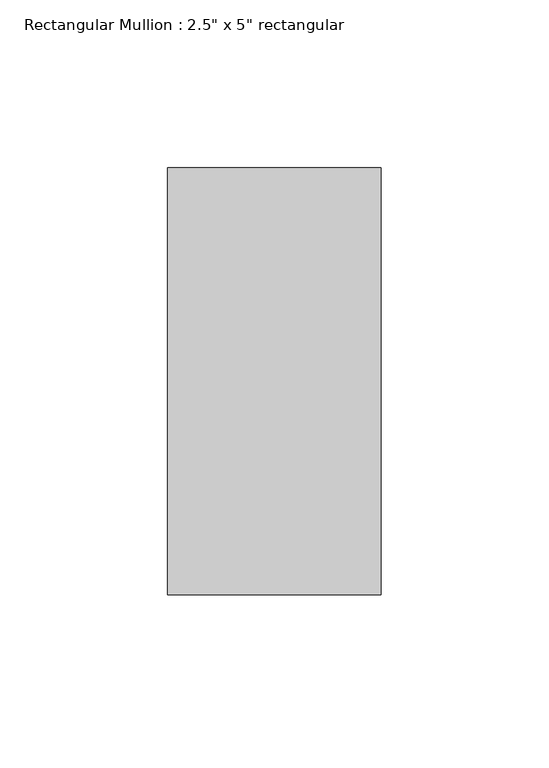
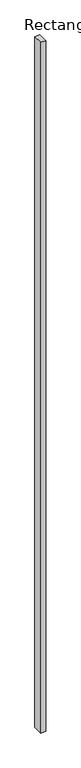
"""IFC4 building model written with IfcOpenShell, lengths in millimetres: member geometry."""

from ifc_helpers import new_model, si_unit, frame, origin, place, context, project, spatial, polyline, outline, extrude, source, transform, mapped, element, save


def member_f5ad0230(model_context):
    return source(origin(), model_context, "Body", "SweptSolid", [
        extrude(outline(polyline([(0.0, 63.5), (0.0, -63.5), (-63.5, -63.5), (-63.5, 63.5), (0.0, 63.5)])), frame((0.0, 0.0, -9130.3702846), z_axis=(0.0, 0.0, 1.0), x_axis=(1.0, 0.0, 0.0)), (0.0, 0.0, 1.0), 9130.3702846),
    ])


if __name__ == "__main__":
    model = new_model("IFC4")
    model_context = context("Model", 3, world=origin())
    ifc_project = project(units=[si_unit("LENGTHUNIT", "METRE", prefix="MILLI")], contexts=[model_context])
    site = spatial("IfcSite", under=ifc_project)
    building = spatial("IfcBuilding", under=site)
    placement = place(None, origin())
    member_shape = member_f5ad0230(model_context)
    element("IfcMember", 1, ObjectType="Rectangular Mullion : 2.5\" x 5\" rectangular", at=placement, inside=building, context=model_context, shape_type="MappedRepresentation", body=[
        mapped(member_shape, transform((0.0, 0.0, 0.0), x_axis=(1.0, 0.0, 0.0), y_axis=(0.0, 1.0, 0.0), z_axis=(0.0, 0.0, 1.0))),
    ])
    save(model, "model.ifc")

# Revit data of these elements
# Type "Rectangular Mullion : 2.5\" x 5\" rectangular"
#   built-in parameter 1007304 = 0.416667 (stored number, unit not read)
#   built-in parameter 1007301 = 0.104167 (stored number, unit not read)
#   built-in parameter 1007300 = 0.104167 (stored number, unit not read)
# Element 1 (IfcMember, "Rectangular Mullion : 2.5\" x 5\" rectangular")
#   Materials on its faces: "Aluminum"
# Materials
#   "Aluminum": class "Metal", colour RGB 247 247 247, transparency 0, Description = "Aluminum 6061", Cost = 0
